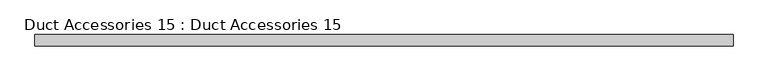
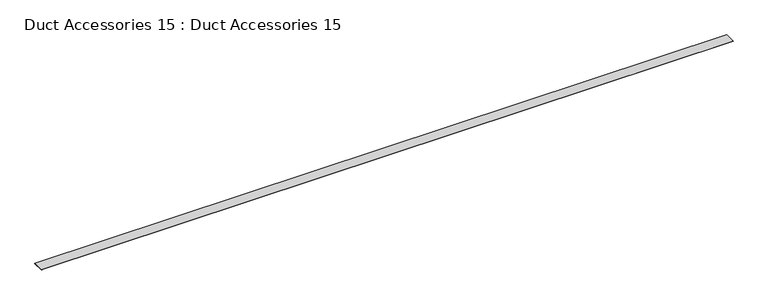
"""IFC4 building model written with IfcOpenShell, lengths in millimetres: damper geometry, Duct Accessories 15 : Duct Accessories 15."""

from ifc_helpers import new_model, si_unit, origin, origin_with_axes, place, context, project, spatial, polyline, outline, extrude, source, transform, mapped, element, save


def duct_accessories_15_duct_accessories_15_503ec04a(model_context):
    return source(origin(), model_context, "Body", "SweptSolid", [
        extrude(outline(polyline([(69053.8278759, -371.2934478), (69053.8278759, -3419.2934478), (-118734.4199308, -3419.2934478), (-118734.4199308, -371.2934478), (69053.8278759, -371.2934478)])), origin_with_axes(), (0.0, 0.0, 1.0), 25.4),
    ])


if __name__ == "__main__":
    model = new_model("IFC4")
    model_context = context("Model", 3, world=origin())
    ifc_project = project(units=[si_unit("LENGTHUNIT", "METRE", prefix="MILLI")], contexts=[model_context])
    site = spatial("IfcSite", under=ifc_project)
    building = spatial("IfcBuilding", under=site)
    placement = place(None, origin())
    duct_accessories_15_duct_accessories_15_shape = duct_accessories_15_duct_accessories_15_503ec04a(model_context)
    element("IfcDamper", 1, ObjectType="Duct Accessories 15 : Duct Accessories 15", at=placement, inside=building, context=model_context, shape_type="MappedRepresentation", body=[
        mapped(duct_accessories_15_duct_accessories_15_shape, transform((0.0, 0.0, 0.0), x_axis=(1.0, 0.0, 0.0), y_axis=(0.0, 1.0, 0.0), z_axis=(0.0, 0.0, 1.0))),
    ])
    save(model, "model.ifc")

# Revit data of these elements
# Element 1 (IfcDamper, "Duct Accessories 15 : Duct Accessories 15")
#   Materials on its faces: "road"
# Materials
#   "road": class "Generic", colour RGB 0 0 0, transparency 0, Cost = 0
